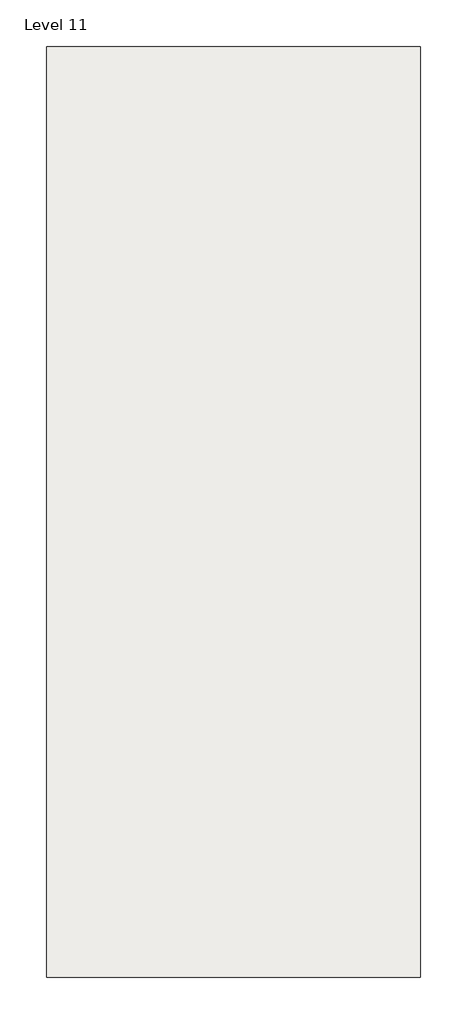
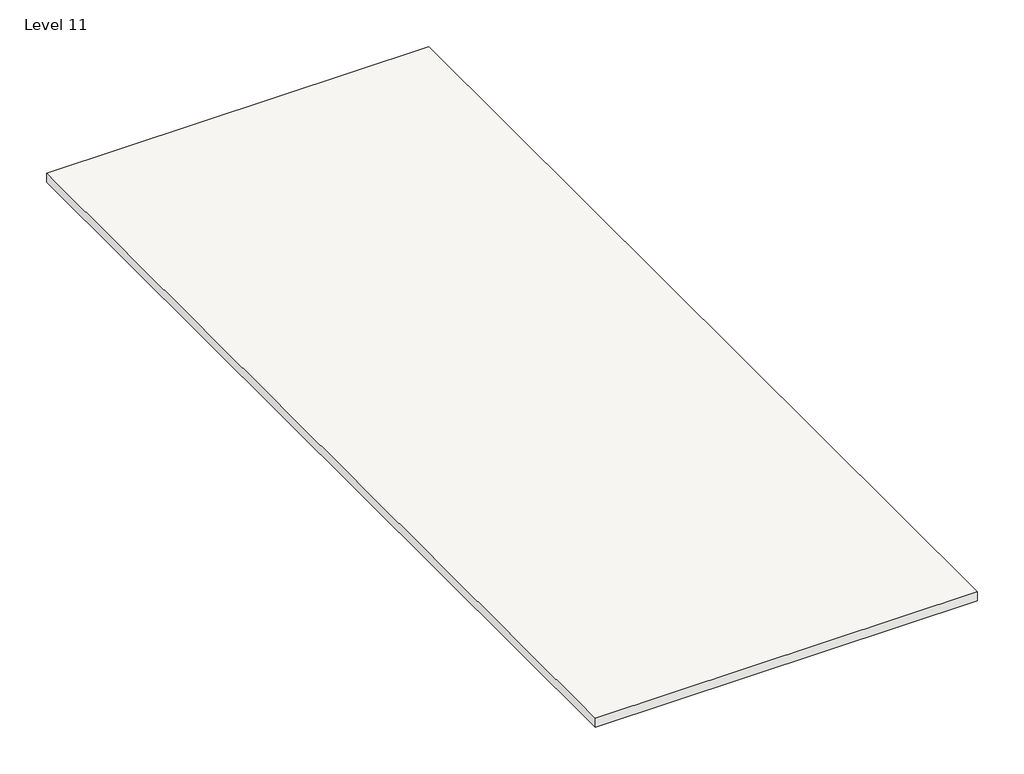
# One storey: 1 slab.
"""IFC4 building model written with IfcOpenShell, lengths in millimetres."""

from ifc_helpers import new_model, si_unit, frame, origin, place, context, project, spatial, polyline, outline, extrude, element, save

model = new_model("IFC4")

# Units and contexts
model_context = context("Model", 3, world=origin())
ifc_project = project(units=[si_unit("LENGTHUNIT", "METRE", prefix="MILLI")], contexts=[model_context])

# Site, building, storey
site = spatial("IfcSite", under=ifc_project)
building = spatial("IfcBuilding", under=site)
storey = spatial("IfcBuildingStorey", under=building, Name="Level 11", Elevation=32004.0)

# Slab
placement = place(None, origin())
element("IfcSlab", 1, ObjectType="Generic - 12\" - Filled", at=placement, inside=storey, context=model_context, shape_type="SweptSolid", body=[
    extrude(outline(polyline([(-376.6902461, 15305.0710592), (-376.6902461, -15403.5289408), (-12721.0902461, -15403.5289408), (-12721.0902461, 15305.0710592), (-376.6902461, 15305.0710592)])), frame((0.0, 0.0, 32004.0), z_axis=(0.0, 0.0, 1.0), x_axis=(1.0, 0.0, 0.0)), (0.0, 0.0, 1.0), 304.8),
])

save(model, "model.ifc")

# Revit data of these elements
# Type "Generic - 12\" - Filled"
#   Assembly Code = "B1010"
#   Function = 0
#   Layers, outside or top first: 1' - 0" no material (function 1)
# Element 1 (IfcSlab, "Generic - 12\" - Filled")
#   Height Offset From Level = 1' - 0"
#   Phase Created = New Construction
#   Materials on its faces: "Default Floor"
# Materials
#   "Default Floor": colour RGB 128 128 128, transparency 0
